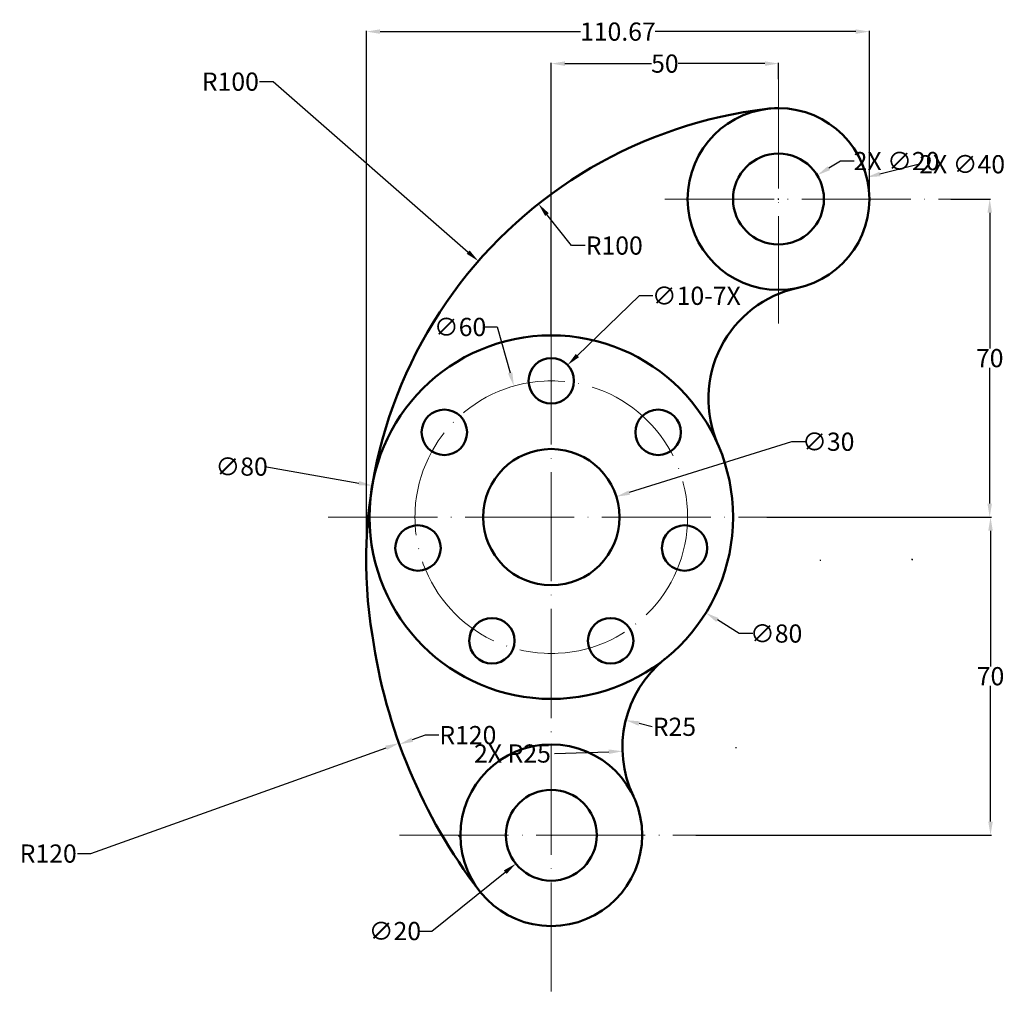
# Model space of a CAD drawing. Units: inches. Extents: x 450 to 667, y 243 to 459.
import ezdxf

# ---------------------------------------------------------------- set-up
doc = ezdxf.new("R2010")
doc.units = ezdxf.units.IN
doc.header["$MEASUREMENT"] = 0
doc.linetypes.add('ACAD_ISO04W100', pattern=[30, 24, -3, 0, -3])
for name, color, linetype, lineweight in [('M-CNTR', 4, 'ACAD_ISO04W100', 18), ('M-DIMS', 2, 'Continuous', 25), ('M-OUTL', 7, 'Continuous', 50)]:
    doc.layers.add(name, color=color, linetype=linetype, lineweight=lineweight)
doc.styles.get("Standard").update_dxf_attribs({"font": 'arial.ttf'})
doc.dimstyles.get("Standard").update_dxf_attribs({"dimtxt": 4, "dimasz": 3, "dimexe": 0.18, "dimexo": 0.0625, "dimgap": 0.09, "dimtad": 0, "dimtih": 1, "dimtoh": 1, "dimdec": 0, "dimzin": 0, "dimdsep": 46, "dimtxsty": 'Standard', "dimcen": 0.09, "dimadec": 0, "dimazin": 0, "dimtfac": 1, "dimtdec": 0, "dimtofl": 0, "dimtmove": 0, "dimatfit": 3, "dimfxl": 1, "dimtolj": 1, "dimtzin": 0, "dimarcsym": 0})

# ---------------------------------------------------------------- blocks, each defined once
blk = doc.blocks.new('*D1')
at = {"layer": 'Defpoints', "color": 0, "transparency": 16777216}
for p in [(617.08, 449.62), (617.08, 446.15), (567.08, 389.81)]:
    blk.add_point(p, dxfattribs=at)
at = {"layer": 'M-DIMS', "color": 0, "lineweight": -2, "transparency": 16777216}
for p, q in [((567.08, 389.87), (567.08, 449.8)), ((570.08, 449.62), (589.13, 449.62)), ((614.08, 449.62), (595.03, 449.62)), ((617.08, 446.21), (617.08, 449.8))]:
    blk.add_line(p, q, dxfattribs=at)
at = {"layer": 'M-DIMS', "color": 0, "transparency": 16777216}
for points in [[(570.08, 450.12), (570.08, 449.12), (567.08, 449.62)], [(614.08, 450.12), (614.08, 449.12), (617.08, 449.62)]]:
    blk.add_solid(points, dxfattribs=at)
at = {"layer": 'M-DIMS', "color": 0, "transparency": 16777216, "insert": (592.08, 449.62), "char_height": 4, "attachment_point": 5}
blk.add_mtext('\\A1;50', dxfattribs=at)
blk = doc.blocks.new('*D2')
at = {"layer": 'Defpoints', "color": 0, "transparency": 16777216}
for p in [(564.26, 418.75), (626.33, 340.35)]:
    blk.add_point(p, dxfattribs=at)
at = {"layer": 'M-DIMS', "color": 0, "lineweight": -2, "transparency": 16777216}
for p, q in [((571.52, 409.58), (566.12, 416.4)), ((574.52, 409.58), (571.52, 409.58))]:
    blk.add_line(p, q, dxfattribs=at)
at = {"layer": 'M-DIMS', "color": 0, "transparency": 16777216}
blk.add_solid([(566.52, 416.71), (565.73, 416.09), (564.26, 418.75)], dxfattribs=at)
at = {"layer": 'M-DIMS', "color": 0, "transparency": 16777216, "insert": (580.94, 409.58), "char_height": 4, "attachment_point": 5}
blk.add_mtext('\\A1;R100', dxfattribs=at)
blk = doc.blocks.new('*D3')
at = {"layer": 'Defpoints', "color": 0, "transparency": 16777216}
for p in [(558.85, 378.66), (575.31, 320.96)]:
    blk.add_point(p, dxfattribs=at)
at = {"layer": 'M-DIMS', "color": 0, "lineweight": -2, "transparency": 16777216}
for p, q in [((552.14, 391.66), (555.14, 391.66)), ((555.14, 391.66), (558.02, 381.54)), ((566.99, 349.81), (567.17, 349.81)), ((567.08, 349.72), (567.08, 349.9))]:
    blk.add_line(p, q, dxfattribs=at)
at = {"layer": 'M-DIMS', "color": 0, "transparency": 16777216}
blk.add_solid([(558.51, 381.68), (557.54, 381.41), (558.85, 378.66)], dxfattribs=at)
at = {"layer": 'M-DIMS', "color": 0, "transparency": 16777216, "insert": (547.01, 391.66), "char_height": 4, "attachment_point": 5}
blk.add_mtext('\\A1;∅60', dxfattribs=at)
blk = doc.blocks.new('*D4')
at = {"layer": 'Defpoints', "color": 0, "transparency": 16777216}
for p in [(646.54, 340.52), (533.66, 299.81)]:
    blk.add_point(p, dxfattribs=at)
at = {"layer": 'M-DIMS', "color": 0, "lineweight": -2, "transparency": 16777216}
for p, q in [((539.3, 301.85), (536.48, 300.83)), ((542.3, 301.85), (539.3, 301.85))]:
    blk.add_line(p, q, dxfattribs=at)
at = {"layer": 'M-DIMS', "color": 0, "transparency": 16777216}
blk.add_solid([(536.31, 301.3), (536.65, 300.36), (533.66, 299.81)], dxfattribs=at)
at = {"layer": 'M-DIMS', "color": 0, "transparency": 16777216, "insert": (548.72, 301.85), "char_height": 4, "attachment_point": 5}
blk.add_mtext('\\A1;R120', dxfattribs=at)
blk = doc.blocks.new('*D5')
at = {"layer": 'Defpoints', "color": 0, "transparency": 16777216}
for p in [(583.48, 305.13), (607.74, 299.1)]:
    blk.add_point(p, dxfattribs=at)
at = {"layer": 'M-DIMS', "color": 0, "lineweight": -2, "transparency": 16777216}
blk.add_line((589.3, 303.68), (586.39, 304.4), dxfattribs=at)
at = {"layer": 'M-DIMS', "color": 0, "transparency": 16777216}
blk.add_solid([(586.51, 304.89), (586.27, 303.92), (583.48, 305.13)], dxfattribs=at)
at = {"layer": 'M-DIMS', "color": 0, "transparency": 16777216, "insert": (594.18, 303.68), "char_height": 4, "attachment_point": 5}
blk.add_mtext('\\A1;R25', dxfattribs=at)
blk = doc.blocks.new('*D6')
at = {"layer": 'Defpoints', "color": 0, "transparency": 16777216}
for p in [(654.92, 419.81), (614.47, 349.81), (663.57, 349.81)]:
    blk.add_point(p, dxfattribs=at)
at = {"layer": 'M-DIMS', "color": 0, "lineweight": -2, "transparency": 16777216}
for p, q in [((654.98, 419.81), (663.75, 419.81)), ((663.57, 416.81), (663.57, 386.94)), ((663.57, 352.81), (663.57, 382.68)), ((614.54, 349.81), (663.75, 349.81))]:
    blk.add_line(p, q, dxfattribs=at)
at = {"layer": 'M-DIMS', "color": 0, "transparency": 16777216}
for points in [[(663.07, 416.81), (664.07, 416.81), (663.57, 419.81)], [(663.07, 352.81), (664.07, 352.81), (663.57, 349.81)]]:
    blk.add_solid(points, dxfattribs=at)
at = {"layer": 'M-DIMS', "color": 0, "transparency": 16777216, "insert": (663.57, 384.81), "char_height": 4, "attachment_point": 5}
blk.add_mtext('\\A1;70', dxfattribs=at)
blk = doc.blocks.new('*D7')
at = {"layer": 'Defpoints', "color": 0, "transparency": 16777216}
for p in [(614.47, 349.81), (663.75, 349.81), (598.82, 279.81)]:
    blk.add_point(p, dxfattribs=at)
at = {"layer": 'M-DIMS', "color": 0, "lineweight": -2, "transparency": 16777216}
for p, q in [((614.54, 349.81), (663.93, 349.81)), ((663.75, 346.81), (663.75, 316.94)), ((663.75, 282.81), (663.75, 312.68)), ((598.89, 279.81), (663.93, 279.81))]:
    blk.add_line(p, q, dxfattribs=at)
at = {"layer": 'M-DIMS', "color": 0, "transparency": 16777216}
for points in [[(663.25, 346.81), (664.25, 346.81), (663.75, 349.81)], [(663.25, 282.81), (664.25, 282.81), (663.75, 279.81)]]:
    blk.add_solid(points, dxfattribs=at)
at = {"layer": 'M-DIMS', "color": 0, "transparency": 16777216, "insert": (663.75, 314.81), "char_height": 4, "attachment_point": 5}
blk.add_mtext('\\A1;70', dxfattribs=at)
blk = doc.blocks.new('*D8')
at = {"layer": 'Defpoints', "color": 0, "transparency": 16777216}
for p in [(574.88, 286.07), (559.28, 273.55)]:
    blk.add_point(p, dxfattribs=at)
at = {"layer": 'M-DIMS', "color": 0, "lineweight": -2, "transparency": 16777216}
for p, q in [((566.99, 279.81), (567.17, 279.81)), ((567.08, 279.72), (567.08, 279.9)), ((540.8, 258.73), (556.94, 271.68)), ((537.8, 258.73), (540.8, 258.73))]:
    blk.add_line(p, q, dxfattribs=at)
at = {"layer": 'M-DIMS', "color": 0, "transparency": 16777216}
blk.add_solid([(556.63, 272.07), (557.25, 271.29), (559.28, 273.55)], dxfattribs=at)
at = {"layer": 'M-DIMS', "color": 0, "transparency": 16777216, "insert": (532.67, 258.73), "char_height": 4, "attachment_point": 5}
blk.add_mtext('\\A1;∅20', dxfattribs=at)
blk = doc.blocks.new('*D9')
at = {"layer": 'Defpoints', "color": 0, "transparency": 16777216}
for p in [(570.67, 383.29), (563.49, 376.33)]:
    blk.add_point(p, dxfattribs=at)
at = {"layer": 'M-DIMS', "color": 0, "lineweight": -2, "transparency": 16777216}
for p, q in [((586.42, 398.52), (572.83, 385.37)), ((589.42, 398.52), (586.42, 398.52)), ((566.99, 379.81), (567.17, 379.81)), ((567.08, 379.72), (567.08, 379.9))]:
    blk.add_line(p, q, dxfattribs=at)
at = {"layer": 'M-DIMS', "color": 0, "transparency": 16777216}
blk.add_solid([(572.48, 385.73), (573.18, 385.01), (570.67, 383.29)], dxfattribs=at)
at = {"layer": 'M-DIMS', "color": 0, "transparency": 16777216, "insert": (599, 398.52), "char_height": 4, "attachment_point": 5}
blk.add_mtext('\\A1;∅10-7X', dxfattribs=at)
blk = doc.blocks.new('*U10')
blk.add_circle((0, 0), 5)
blk = doc.blocks.new('*U11')
at = {"layer": 'M-OUTL', "color": 0, "linetype": 'ByBlock', "lineweight": -2, "transparency": 16777216}
blk.add_blockref('*U10', (567.08, 379.81), dxfattribs=at)
for p, rotation in [((543.55, 368.48), 51.42857142857145), ((590.6, 368.48), 308.5714285714285), ((537.74, 343.02), 102.8571428571429), ((596.42, 343.02), 257.1428571428572), ((554.02, 322.61), 154.2857142857143), ((580.14, 322.61), 205.7142857142857)]:
    blk.add_blockref('*U10', p, dxfattribs=dict(at, rotation=rotation))
blk = doc.blocks.new('*D12')
at = {"layer": 'Defpoints', "color": 0, "transparency": 16777216}
for p in [(581.39, 354.31), (552.77, 345.31)]:
    blk.add_point(p, dxfattribs=at)
at = {"layer": 'M-DIMS', "color": 0, "lineweight": -2, "transparency": 16777216}
for p, q in [((619.92, 366.41), (584.25, 355.21)), ((622.92, 366.41), (619.92, 366.41)), ((566.99, 349.81), (567.17, 349.81)), ((567.08, 349.72), (567.08, 349.9))]:
    blk.add_line(p, q, dxfattribs=at)
at = {"layer": 'M-DIMS', "color": 0, "transparency": 16777216}
blk.add_solid([(584.1, 355.68), (584.4, 354.73), (581.39, 354.31)], dxfattribs=at)
at = {"layer": 'M-DIMS', "color": 0, "transparency": 16777216, "insert": (628.04, 366.41), "char_height": 4, "attachment_point": 5}
blk.add_mtext('\\A1;∅30', dxfattribs=at)
blk = doc.blocks.new('*D13')
at = {"layer": 'Defpoints', "color": 0, "transparency": 16777216}
for p in [(533.07, 370.86), (601.09, 328.76)]:
    blk.add_point(p, dxfattribs=at)
at = {"layer": 'M-DIMS', "color": 0, "lineweight": -2, "transparency": 16777216}
for p, q in [((566.99, 349.81), (567.17, 349.81)), ((567.08, 349.72), (567.08, 349.9)), ((608.45, 324.2), (603.64, 327.18)), ((611.45, 324.2), (608.45, 324.2))]:
    blk.add_line(p, q, dxfattribs=at)
at = {"layer": 'M-DIMS', "color": 0, "transparency": 16777216}
blk.add_solid([(603.9, 327.6), (603.38, 326.75), (601.09, 328.76)], dxfattribs=at)
at = {"layer": 'M-DIMS', "color": 0, "transparency": 16777216, "insert": (616.57, 324.2), "char_height": 4, "attachment_point": 5}
blk.add_mtext('\\A1;∅80', dxfattribs=at)
blk = doc.blocks.new('LINK-EYE-40-20')
for radius in [20, 10]:
    blk.add_circle((0, 0), radius)
blk = doc.blocks.new('*D15')
at = {"layer": 'Defpoints', "color": 0, "transparency": 16777216}
for p in [(637.08, 456.66), (637.08, 419.81), (526.41, 344.29)]:
    blk.add_point(p, dxfattribs=at)
at = {"layer": 'M-DIMS', "color": 0, "lineweight": -2, "transparency": 16777216}
for p, q in [((526.41, 344.35), (526.41, 456.84)), ((529.41, 456.66), (573.54, 456.66)), ((634.08, 456.66), (589.95, 456.66)), ((637.08, 419.87), (637.08, 456.84))]:
    blk.add_line(p, q, dxfattribs=at)
at = {"layer": 'M-DIMS', "color": 0, "transparency": 16777216}
for points in [[(529.41, 457.16), (529.41, 456.16), (526.41, 456.66)], [(634.08, 457.16), (634.08, 456.16), (637.08, 456.66)]]:
    blk.add_solid(points, dxfattribs=at)
at = {"layer": 'M-DIMS', "color": 0, "transparency": 16777216, "insert": (581.74, 456.66), "char_height": 4, "attachment_point": 5}
blk.add_mtext('\\A1;110.67', dxfattribs=at)
blk = doc.blocks.new('*D16')
at = {"layer": 'Defpoints', "color": 0, "transparency": 16777216}
for p in [(636.5, 424.6), (597.66, 415.02)]:
    blk.add_point(p, dxfattribs=at)
at = {"layer": 'M-DIMS', "color": 0, "lineweight": -2, "transparency": 16777216}
for p, q in [((648.15, 427.47), (639.41, 425.32)), ((616.99, 419.81), (617.17, 419.81)), ((617.08, 419.72), (617.08, 419.9))]:
    blk.add_line(p, q, dxfattribs=at)
at = {"layer": 'M-DIMS', "color": 0, "transparency": 16777216}
blk.add_solid([(639.29, 425.8), (639.53, 424.83), (636.5, 424.6)], dxfattribs=at)
at = {"layer": 'M-DIMS', "color": 0, "transparency": 16777216, "insert": (657.5, 427.47), "char_height": 4, "attachment_point": 5}
blk.add_mtext('\\A1;2X ∅40', dxfattribs=at)
blk = doc.blocks.new('*D17')
at = {"layer": 'Defpoints', "color": 0, "transparency": 16777216}
for p in [(625.6, 425.04), (608.55, 414.58)]:
    blk.add_point(p, dxfattribs=at)
at = {"layer": 'M-DIMS', "color": 0, "lineweight": -2, "transparency": 16777216}
for p, q in [((630.72, 428.17), (628.16, 426.6)), ((633.72, 428.17), (630.72, 428.17)), ((616.99, 419.81), (617.17, 419.81)), ((617.08, 419.72), (617.08, 419.9))]:
    blk.add_line(p, q, dxfattribs=at)
at = {"layer": 'M-DIMS', "color": 0, "transparency": 16777216}
blk.add_solid([(627.9, 427.03), (628.42, 426.18), (625.6, 425.04)], dxfattribs=at)
at = {"layer": 'M-DIMS', "color": 0, "transparency": 16777216, "insert": (643.07, 428.17), "char_height": 4, "attachment_point": 5}
blk.add_mtext('\\A1;2X ∅20', dxfattribs=at)
blk = doc.blocks.new('*D18')
at = {"layer": 'Defpoints', "color": 0, "transparency": 16777216}
for p in [(551.04, 406.16), (626.33, 340.35)]:
    blk.add_point(p, dxfattribs=at)
at = {"layer": 'M-DIMS', "color": 0, "lineweight": -2, "transparency": 16777216}
for p, q in [((502.87, 445.65), (505.87, 445.65)), ((505.87, 445.65), (548.78, 408.14)), ((626.24, 340.35), (626.42, 340.35)), ((626.33, 340.26), (626.33, 340.44))]:
    blk.add_line(p, q, dxfattribs=at)
at = {"layer": 'M-DIMS', "color": 0, "transparency": 16777216}
blk.add_solid([(549.11, 408.51), (548.45, 407.76), (551.04, 406.16)], dxfattribs=at)
at = {"layer": 'M-DIMS', "color": 0, "transparency": 16777216, "insert": (496.45, 445.65), "char_height": 4, "attachment_point": 5}
blk.add_mtext('\\A1;R100', dxfattribs=at)
blk = doc.blocks.new('*D19')
at = {"layer": 'Defpoints', "color": 0, "transparency": 16777216}
for p in [(646.54, 340.52), (533.57, 300.06)]:
    blk.add_point(p, dxfattribs=at)
at = {"layer": 'M-DIMS', "color": 0, "lineweight": -2, "transparency": 16777216}
for p, q in [((646.45, 340.52), (646.63, 340.52)), ((646.54, 340.43), (646.54, 340.61)), ((465.78, 275.78), (530.74, 299.05)), ((462.78, 275.78), (465.78, 275.78))]:
    blk.add_line(p, q, dxfattribs=at)
at = {"layer": 'M-DIMS', "color": 0, "transparency": 16777216}
blk.add_solid([(530.57, 299.52), (530.91, 298.58), (533.57, 300.06)], dxfattribs=at)
at = {"layer": 'M-DIMS', "color": 0, "transparency": 16777216, "insert": (456.37, 275.78), "char_height": 4, "attachment_point": 5}
blk.add_mtext('\\A1;R120', dxfattribs=at)
blk = doc.blocks.new('*D20')
at = {"layer": 'Defpoints', "color": 0, "transparency": 16777216}
for p in [(607.74, 299.1), (582.75, 298.29)]:
    blk.add_point(p, dxfattribs=at)
at = {"layer": 'M-DIMS', "color": 0, "lineweight": -2, "transparency": 16777216}
for p, q in [((607.65, 299.1), (607.83, 299.1)), ((607.74, 299.01), (607.74, 299.19)), ((567.76, 297.8), (579.75, 298.19))]:
    blk.add_line(p, q, dxfattribs=at)
at = {"layer": 'M-DIMS', "color": 0, "transparency": 16777216}
blk.add_solid([(579.74, 298.69), (579.77, 297.69), (582.75, 298.29)], dxfattribs=at)
at = {"layer": 'M-DIMS', "color": 0, "transparency": 16777216, "insert": (558.54, 297.8), "char_height": 4, "attachment_point": 5}
blk.add_mtext('\\A1;2X R25', dxfattribs=at)
blk = doc.blocks.new('*D21')
at = {"layer": 'Defpoints', "color": 0, "transparency": 16777216}
for p in [(527.69, 356.76), (606.47, 342.86)]:
    blk.add_point(p, dxfattribs=at)
at = {"layer": 'M-DIMS', "color": 0, "lineweight": -2, "transparency": 16777216}
for p, q in [((504.05, 360.93), (524.73, 357.28)), ((566.99, 349.81), (567.17, 349.81)), ((567.08, 349.72), (567.08, 349.9))]:
    blk.add_line(p, q, dxfattribs=at)
at = {"layer": 'M-DIMS', "color": 0, "transparency": 16777216}
blk.add_solid([(524.82, 357.77), (524.65, 356.79), (527.69, 356.76)], dxfattribs=at)
at = {"layer": 'M-DIMS', "color": 0, "transparency": 16777216, "insert": (498.93, 360.93), "char_height": 4, "attachment_point": 5}
blk.add_mtext('\\A1;∅80', dxfattribs=at)

msp = doc.modelspace()

# ---------------------------------------------------------------- linework, layer by layer
at = {"layer": 'M-CNTR'}
for p, q in [((617.08, 446.146), (617.08, 392.421)), ((592.103, 419.81), (654.916, 419.81)), ((567.08, 389.81), (567.08, 243.048)), ((518.009, 349.81), (614.475, 349.81)), ((533.668, 279.81), (598.825, 279.81))]:
    msp.add_line(p, q, dxfattribs=at)
msp.add_circle((567.08, 349.81), 30, dxfattribs=at)
at = {"layer": 'M-OUTL'}
for radius in [40, 15]:
    msp.add_circle((567.08, 349.81), radius, dxfattribs=at)
for centre, radius, start, end in [((626.329, 340.347), 100, 95.30686, 189.58862), ((626.641, 375.838), 25, 102.26755, 203.60466), ((646.539, 340.524), 120, 188.06478, 217.3832), ((607.737, 299.096), 25, 128.7193, 205.37693), ((626.329, 340.347), 100, 217.25507, 217.58615), ((626.329, 340.347), 100, 233.64545, 233.66611)]:
    msp.add_arc(centre, radius, start, end, dxfattribs=at)

# ---------------------------------------------------------------- block references
for name, p in [('LINK-EYE-40-20', (617.08, 419.81)), ('*U11', (0, 0)), ('LINK-EYE-40-20', (567.08, 279.81))]:
    msp.add_blockref(name, p, dxfattribs=at)

# ---------------------------------------------------------------- dimensions: what is measured, and where the dimension line sits
at = {"layer": 'M-DIMS'}
for base, p1, p2, override, picture, middle in [((637.08, 456.656), (526.406, 344.286), (637.08, 419.81), {"dimdec": 2, "dimlfac": 1, "dimrnd": 0, "dimzin": 0, "dimdsep": 46, "dimlunit": 2}, '*D15', (581.743, 456.656)), ((617.08, 449.615), (567.08, 389.81), (617.08, 446.146), {"dimclrd": 0, "dimclre": 0, "dimclrt": 0}, '*D1', (592.08, 449.615))]:
    dim = msp.add_linear_dim(base=base, p1=p1, p2=p2, dimstyle='Standard', override=override, dxfattribs=at)
    dim.commit()
    dim.dimension.update_dxf_attribs({"geometry": picture, "text_midpoint": middle})
for center, mpoint, override, picture, middle in [((626.329, 340.347), (551.042, 406.164), {"dimdec": 0, "dimlfac": 1, "dimrnd": 0, "dimzin": 0, "dimdsep": 46, "dimlunit": 2}, '*D18', (496.453, 445.654)), ((626.329, 340.347), (564.262, 418.754), {"dimclrd": 0, "dimclre": 0, "dimclrt": 0}, '*D2', (580.937, 409.584)), ((646.539, 340.524), (533.567, 300.06), {"dimdec": 0, "dimlfac": 1, "dimrnd": 0, "dimzin": 0, "dimdsep": 46, "dimlunit": 2}, '*D19', (456.368, 275.781)), ((646.539, 340.524), (533.655, 299.814), {"dimclrd": 0, "dimclre": 0, "dimclrt": 0}, '*D4', (548.716, 301.85)), ((607.737, 299.096), (583.476, 305.127), {"dimclrd": 0, "dimclre": 0, "dimclrt": 0}, '*D5', (589.299, 303.68))]:
    dim = msp.add_radius_dim(center=center, mpoint=mpoint, dimstyle='Standard', override=override, dxfattribs=at)
    dim.commit()
    dim.dimension.update_dxf_attribs({"geometry": picture, "text_midpoint": middle, "dimtype": 164})
for p1, p2, text, override, picture, middle in [((597.661, 415.021), (636.498, 424.599), '2X <>', {"dimdec": 0, "dimlfac": 1, "dimrnd": 0, "dimzin": 0, "dimdsep": 46, "dimlunit": 2}, '*D16', (648.149, 427.473)), ((608.554, 414.583), (625.605, 425.037), '2X <>', {"dimdec": 0, "dimlfac": 1, "dimrnd": 0, "dimzin": 0, "dimdsep": 46, "dimlunit": 2}, '*D17', (643.069, 428.173)), ((563.487, 376.333), (570.673, 383.287), '<>-7X', {"dimclrd": 0, "dimclre": 0, "dimclrt": 0}, '*D9', (599.005, 398.525))]:
    dim = msp.add_diameter_dim_2p(p1=p1, p2=p2, text=text, dimstyle='Standard', override=override, dxfattribs=at)
    dim.commit()
    dim.dimension.update_dxf_attribs({"geometry": picture, "text_midpoint": middle, "dimtype": 163})
for base, p1, picture, middle in [((663.573, 349.81), (654.916, 419.81), '*D6', (663.573, 384.81)), ((663.753, 349.81), (598.825, 279.81), '*D7', (663.753, 314.81))]:
    dim = msp.add_linear_dim(base=base, p1=p1, p2=(614.475, 349.81), angle=90, dimstyle='Standard', override={"dimclrd": 0, "dimclre": 0, "dimclrt": 0}, dxfattribs=at)
    dim.commit()
    dim.dimension.update_dxf_attribs({"geometry": picture, "text_midpoint": middle})
for p1, p2, override, picture, middle in [((575.311, 320.962), (558.848, 378.659), {"dimclrd": 0, "dimclre": 0, "dimclrt": 0}, '*D3', (547.013, 391.661)), ((533.069, 370.864), (601.09, 328.756), {"dimclrd": 0, "dimclre": 0, "dimclrt": 0}, '*D13', (616.572, 324.202)), ((552.769, 345.314), (581.39, 354.307), {"dimclrd": 0, "dimclre": 0, "dimclrt": 0}, '*D12', (628.045, 366.413)), ((606.471, 342.86), (527.688, 356.76), {"dimdec": 0, "dimlfac": 1, "dimrnd": 0, "dimzin": 0, "dimdsep": 46, "dimlunit": 2}, '*D21', (504.053, 360.93)), ((574.88, 286.068), (559.279, 273.553), {"dimclrd": 0, "dimclre": 0, "dimclrt": 0}, '*D8', (532.675, 258.727))]:
    dim = msp.add_diameter_dim_2p(p1=p1, p2=p2, dimstyle='Standard', override=override, dxfattribs=at)
    dim.commit()
    dim.dimension.update_dxf_attribs({"geometry": picture, "text_midpoint": middle, "dimtype": 163})
dim = msp.add_radius_dim(center=(607.737, 299.096), mpoint=(582.75, 298.289), text='2X <>', dimstyle='Standard', override={"dimdec": 0, "dimlfac": 1, "dimrnd": 0, "dimzin": 0, "dimdsep": 46, "dimlunit": 2}, dxfattribs=at)
dim.commit()
dim.dimension.update_dxf_attribs({"geometry": '*D20', "text_midpoint": (567.758, 297.804), "dimtype": 164})

doc.saveas('drawing.dxf')
